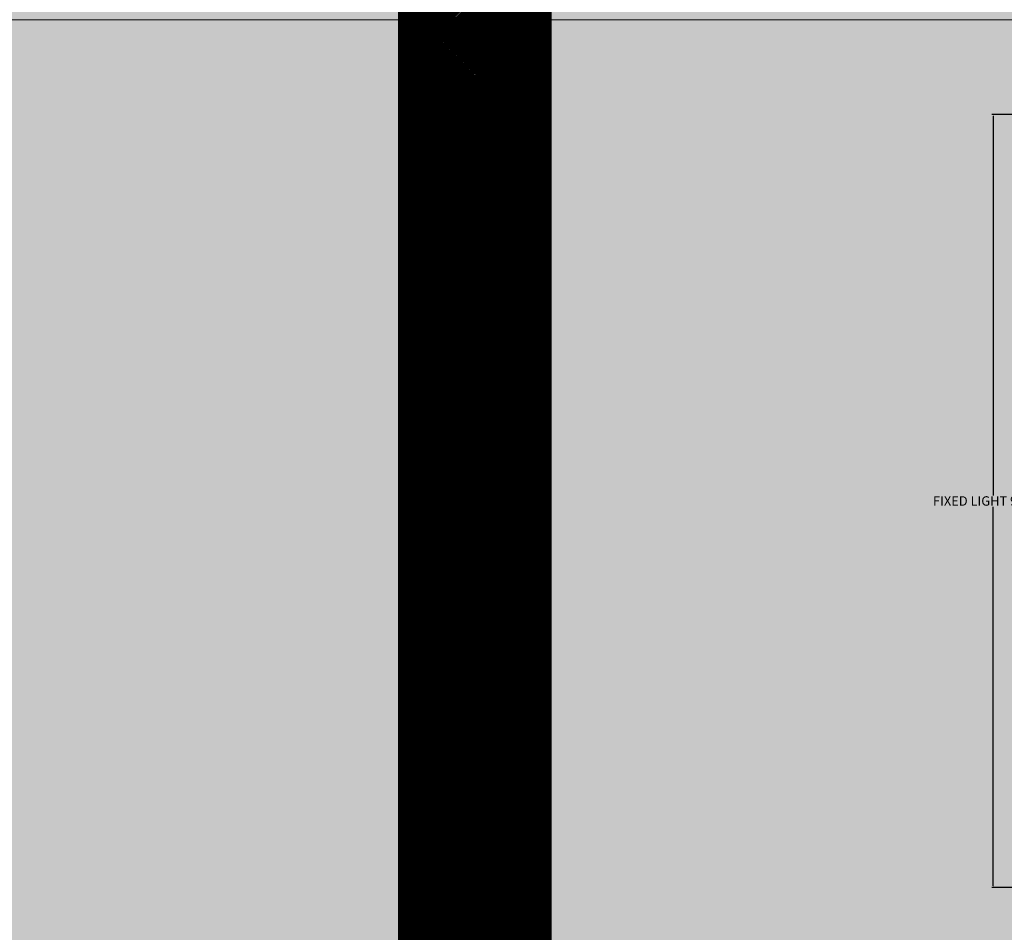
# Model space of a CAD drawing. Units: inches. Extents: x 8 to 634, y 41 to 867.
# Tile 10 of 21: x 297 to 415, y 283 to 392. Entities that reach past the tile are written whole.
import ezdxf

# ---------------------------------------------------------------- set-up
doc = ezdxf.new("R2010")
doc.units = ezdxf.units.IN
doc.header["$MEASUREMENT"] = 0
for name, color, linetype, lineweight in [('A-ANNO-DIMS', 2, 'Continuous', 18), ('A-ELEV-PATT', 252, 'Continuous', 9), ('A-WALL', 7, 'Continuous', 35), ('A-WALL-PANL', 7, 'Continuous', 18), ('A-WALL-PATT', 8, 'Continuous', 9)]:
    doc.layers.add(name, color=color, linetype=linetype, lineweight=lineweight)
doc.styles.get("Standard").update_dxf_attribs({"font": 'arial.ttf'})
doc.dimstyles.get("Standard").update_dxf_attribs({"dimtxt": 1.125, "dimasz": 0.18, "dimexe": 0.18, "dimexo": 0.0625, "dimgap": 0.09, "dimtad": 0, "dimtih": 1, "dimtoh": 1, "dimdec": 4, "dimzin": 0, "dimdsep": 46, "dimlunit": 4, "dimtxsty": 'Standard', "dimcen": 0.09, "dimadec": 0, "dimazin": 0, "dimtfac": 1, "dimtdec": 4, "dimtofl": 0, "dimtmove": 0, "dimatfit": 3, "dimfxl": 1, "dimtolj": 1, "dimtzin": 0, "dimarcsym": 0})

# ---------------------------------------------------------------- blocks, each defined once
blk = doc.blocks.new('*D7')
at = {"layer": 'A-ANNO-DIMS', "color": 0, "lineweight": -2, "transparency": 16777216}
for p, q in [((427.37, 380.43), (413.42, 380.43)), ((413.6, 380.25), (413.6, 334.97)), ((413.6, 288.35), (413.6, 333.62)), ((427.37, 288.17), (413.42, 288.17))]:
    blk.add_line(p, q, dxfattribs=at)
at = {"layer": 'A-ANNO-DIMS', "color": 0, "transparency": 16777216}
for points in [[(413.57, 380.25), (413.63, 380.25), (413.6, 380.43)], [(413.57, 288.35), (413.63, 288.35), (413.6, 288.17)]]:
    blk.add_solid(points, dxfattribs=at)
at = {"layer": 'Defpoints', "color": 0, "transparency": 16777216}
for p in [(413.6, 380.43), (427.44, 380.43), (427.44, 288.17)]:
    blk.add_point(p, dxfattribs=at)
at = {"layer": 'A-ANNO-DIMS', "color": 0, "transparency": 16777216, "insert": (413.6, 334.3), "char_height": 1.125, "attachment_point": 5}
blk.add_mtext('\\A1;FIXED LIGHT 92 TYP.', dxfattribs=at)

msp = doc.modelspace()

# ---------------------------------------------------------------- hatches: boundary and pattern name
at = {"layer": 'A-ELEV-PATT', "transparency": 33554544}
h = msp.add_hatch(dxfattribs=at)
h.set_pattern_fill('ANSI31', color=256)
h.paths.add_polyline_path([(360.785, 697.6655), (342.6544, 682.1444), (342.6544, 569.1705), (360.785, 569.1705)])
h.paths.add_polyline_path([(360.785, 523.5555), (360.785, 569.1705), (342.6544, 569.1705), (342.6544, 449.7533), (360.785, 449.7533)])
h.paths.add_polyline_path([(360.785, 449.7533), (342.6544, 449.7533), (342.6544, 391.7598), (360.785, 391.7598)])
h.paths.add_polyline_path([(360.785, 391.7598), (342.6544, 391.7598), (342.6544, 272.3426), (360.785, 272.3426)])
h.paths.add_polyline_path([(360.785, 272.3426), (342.6544, 272.3426), (342.6544, 235.5555), (360.785, 235.5555)])
h.paths.add_polyline_path([(360.785, 235.5555), (342.6544, 235.5555), (342.6544, 224.3257), (353.4573, 224.3257), (353.4573, 101.0012), (342.6544, 101.0012), (342.6544, 91.5417), (360.785, 91.5417)])
at = {"layer": 'A-WALL-PATT', "transparency": 33554687}
h = msp.add_hatch(dxfattribs=at)
h.set_pattern_fill('AR-CONC', color=256, scale=3.2)
h.paths.add_polyline_path([(119.7065, 697.6655), (47.3401, 697.6655), (47.3401, 569.1705), (119.7065, 569.1705)])
h.paths.add_polyline_path([(202.1558, 697.6655), (119.7065, 697.6655), (119.7065, 569.1705), (202.1558, 569.1705)])
h.paths.add_polyline_path([(284.6051, 697.6655), (202.1558, 697.6655), (202.1558, 569.1705), (284.6051, 569.1705)])
h.paths.add_polyline_path([(119.7065, 569.1705), (47.3401, 569.1705), (47.3401, 523.5555), (47.3401, 449.7533), (119.7065, 449.7533)])
h.paths.add_polyline_path([(342.6544, 682.1444), (360.785, 697.6655), (284.6051, 697.6655), (284.6051, 569.1705), (342.6544, 569.1705)])
h.paths.add_polyline_path([(342.6544, 569.1705), (284.6051, 569.1705), (284.6051, 449.7533), (342.6544, 449.7533)])
h.paths.add_polyline_path([(418.2881, 691.978), (418.2881, 697.6655), (360.785, 697.6655), (360.785, 569.1705), (418.2881, 569.1705)])
h.paths.add_polyline_path([(418.2881, 569.1705), (360.785, 569.1705), (360.785, 523.5555), (360.785, 449.7533), (418.2881, 449.7533)])
h.paths.add_polyline_path([(594.3501, 697.6655), (539.0002, 697.6655), (539.0002, 691.978), (539.0002, 569.1705), (594.3501, 569.1705)])
h.paths.add_polyline_path([(594.3501, 523.5555), (594.3501, 569.1705), (539.0002, 569.1705), (539.0002, 451.6305), (594.3501, 451.6305)])
h.paths.add_polyline_path([(594.3501, 451.6305), (539.0002, 451.6305), (539.0002, 391.7598), (594.3501, 391.7598)])
h.paths.add_polyline_path([(594.3501, 391.7598), (539.0002, 391.7598), (539.0002, 276.166), (594.3501, 276.166)])
h.paths.add_polyline_path([(418.2881, 449.7533), (360.785, 449.7533), (360.785, 391.7598), (418.2881, 391.7598)])
h.paths.add_polyline_path([(342.6544, 449.7533), (284.6051, 449.7533), (284.6051, 391.7598), (342.6544, 391.7598)])
h.paths.add_polyline_path([(342.6544, 391.7598), (284.6051, 391.7598), (284.6051, 272.3426), (342.6544, 272.3426)])
h.paths.add_polyline_path([(418.2881, 391.7598), (360.785, 391.7598), (360.785, 272.3426), (418.2881, 272.3426)])
h.paths.add_polyline_path([(418.2881, 272.3426), (360.785, 272.3426), (360.785, 235.5555), (418.2881, 235.5555)])
h.paths.add_polyline_path([(342.6544, 272.3426), (284.6051, 272.3426), (284.6051, 235.5555), (295.0049, 235.5555), (342.6544, 235.5555)])
h.paths.add_polyline_path([(594.3501, 276.166), (539.0002, 276.166), (539.0002, 228.4951), (594.3501, 228.4951)])
h.paths.add_polyline_path([(594.3501, 228.4951), (539.0002, 228.4951), (539.0002, 91.5417), (594.3501, 91.5417)])
h.paths.add_polyline_path([(418.2881, 235.5555), (360.785, 235.5555), (360.785, 91.5417), (418.2881, 91.5417)])
h.paths.add_polyline_path([(284.6051, 272.3426), (119.7065, 272.3426), (119.7065, 235.5555), (284.6051, 235.5555)])
h.paths.add_polyline_path([(119.7065, 272.3426), (47.3401, 272.3426), (47.3401, 235.5555), (47.3401, 91.5555), (63.5448, 91.5555), (63.5448, 227.8036), (268.998, 227.8036), (268.998, 91.5555), (295.0049, 91.5555), (295.0049, 222.583), (271.9787, 222.583), (271.9787, 229.0481), (62.4019, 229.0481), (62.4019, 222.583), (61.1827, 222.583), (61.1827, 235.5555), (119.7065, 235.5555)])
h.paths.add_polyline_path([(119.7065, 391.7598), (47.3401, 391.7598), (47.3401, 379.5555), (47.3401, 272.3426), (119.7065, 272.3426)])
h.paths.add_polyline_path([(119.7065, 449.7533), (47.3401, 449.7533), (47.3401, 391.7598), (119.7065, 391.7598)])
h.paths.add_polyline_path([(202.1558, 449.7533), (119.7065, 449.7533), (119.7065, 391.7598), (202.1558, 391.7598)])
h.paths.add_polyline_path([(284.6051, 449.7533), (202.1558, 449.7533), (202.1558, 391.7598), (284.6051, 391.7598)])

# ---------------------------------------------------------------- linework, layer by layer
at = {"layer": 'A-WALL'}
for p, q in [((342.6544, 682.1444), (342.6544, 91.5555)), ((360.785, 235.5555), (360.785, 523.5555))]:
    msp.add_line(p, q, dxfattribs=at)
at = {"layer": 'A-WALL-PANL'}
msp.add_line((418.2881, 391.7598), (47.3401, 391.7598), dxfattribs=at)

# ---------------------------------------------------------------- dimensions: what is measured, and where the dimension line sits
at = {"layer": 'A-ANNO-DIMS'}
dim = msp.add_linear_dim(base=(413.5977, 380.4268), p1=(427.4368, 288.166), p2=(427.4368, 380.4268), angle=90, text='FIXED LIGHT <> TYP.', dimstyle='Standard', override={"dimdec": 0, "dimlfac": 1, "dimrnd": 0, "dimzin": 0, "dimdsep": 46, "dimlunit": 2}, dxfattribs=at)
dim.commit()
dim.dimension.update_dxf_attribs({"geometry": '*D7', "text_midpoint": (413.5977, 334.2964)})

doc.saveas('drawing.dxf')
